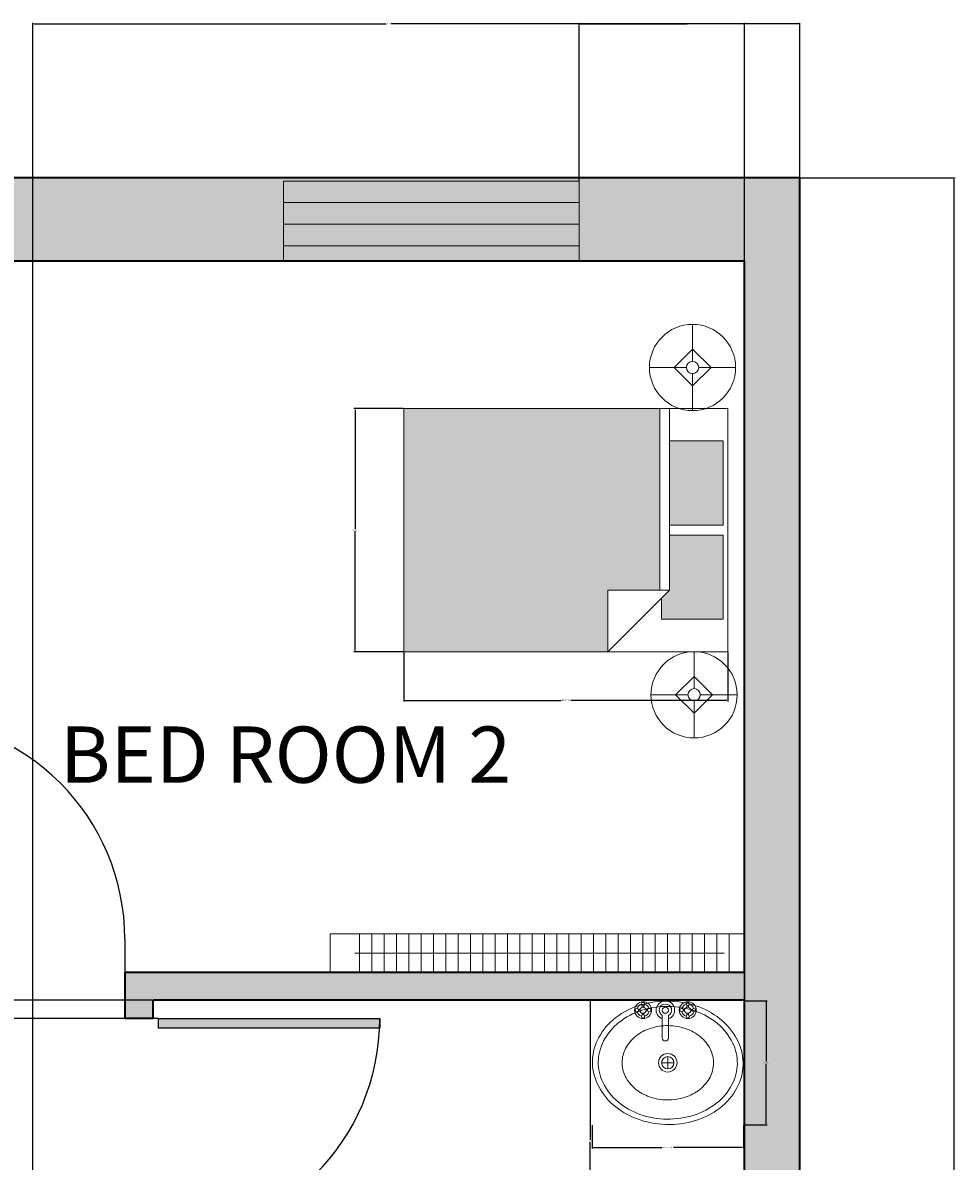
# Model space of a CAD drawing. Units: inches. Extents: x 1434 to 1845, y 1483 to 2014.
# Tile 11 of 11: x 1693 to 1845, y 1829 to 2014. Entities that reach past the tile are written whole.
import ezdxf

# ---------------------------------------------------------------- set-up
doc = ezdxf.new("R2010")
doc.units = ezdxf.units.IN
for name, color, linetype, lineweight in [('A-ANNO-DIMS', 2, 'Continuous', 18), ('A-AREA-IDEN', 7, 'Continuous', 25), ('A-DOOR', 3, 'Continuous', 25), ('A-FLOR-FIXT', 8, 'Continuous', 18), ('A-FLOR-FIXT-PATT', 8, 'Continuous', 13), ('A-FURN', 9, 'Continuous', 18), ('A-FURN-PATT', 9, 'Continuous', 13), ('A-GLAZ', 4, 'Continuous', 18), ('A-GLAZ-PATT', 9, 'Continuous', 13), ('A-WALL', 7, 'Continuous', 35), ('A-WALL-PATT', 8, 'Continuous', 13), ('E-LITE', 2, 'Continuous', 18)]:
    doc.layers.add(name, color=color, linetype=linetype, lineweight=lineweight)
doc.layers.add('A-DOOR-PATT', color=39, linetype='Continuous', lineweight=13, true_color=0x58382b)
doc.styles.get("Standard").update_dxf_attribs({"font": 'arial.ttf'})
doc.dimstyles.get("Standard").update_dxf_attribs({"dimtxt": 0.18, "dimasz": 0.18, "dimexe": 0.18, "dimexo": 0.0625, "dimgap": 0.09, "dimtad": 0, "dimtih": 1, "dimtoh": 1, "dimdec": 4, "dimzin": 0, "dimdsep": 46, "dimtxsty": 'Standard', "dimcen": 0.09, "dimadec": 0, "dimazin": 0, "dimtfac": 1, "dimtdec": 4, "dimtofl": 0, "dimtmove": 0, "dimatfit": 3, "dimfxl": 1, "dimtolj": 1, "dimtzin": 0, "dimarcsym": 0})

# ---------------------------------------------------------------- blocks, each defined once
blk = doc.blocks.new('*U3')
for p, q in [((0, 0), (0, -6)), ((40, 0), (40, -6))]:
    blk.add_line(p, q)
blk.add_lwpolyline([(0, 0), (0, 40), (1.75, 40), (1.75, 0)], close=True)
blk.add_arc((0, 0), 40, 0, 90)
blk = doc.blocks.new('Bed - Queen')
for p, q in [((0, -80.00003), (0, 0)), ((0, 0), (59.99999, 0)), ((59.99999, 0), (59.99999, -80.00003)), ((7.99999, -1.2), (28.79998, -1.2)), ((7.99999, -14.4), (7.99999, -1.2)), ((28.79998, -1.2), (28.79998, -14.4)), ((31.19999, -1.2), (51.99999, -1.2)), ((31.19999, -14.4), (31.19999, -1.2)), ((51.99999, -1.2), (51.99999, -16.4)), ((0, -14.4), (44.8, -14.4)), ((44.8, -16.8), (0, -16.8)), ((59.99999, -29.6), (44.8, -14.4)), ((44.8, -14.4), (44.8, -29.6)), ((51.99999, -16.4), (46.79936, -16.4)), ((44.8, -29.6), (59.99999, -29.6)), ((59.99999, -80.00003), (0, -80.00003))]:
    blk.add_line(p, q)
blk = doc.blocks.new('Lamp - Table')
for p, q in [((0, 7), (0, 1)), ((0, 3), (-3, 0)), ((3, 0), (0, 3)), ((-1, 0), (-7, 0)), ((-3, 0), (0, -3)), ((0, -3), (3, 0)), ((1, 0), (7, 0)), ((0, -1), (0, -7))]:
    blk.add_line(p, q)
for radius in [7, 1]:
    blk.add_circle((0, 0), radius)
blk = doc.blocks.new('Sink - Oval top')
for p, q in [((-1, 0), (1, 0)), ((0, 1), (0, -1))]:
    blk.add_line(p, q)
for points in [[(-12.23, 0.39, 0.117634), (-11.46, -3.36, 0.104469), (-8.88, -6.8, 0.090016), (-5.08, -9.07, 0.08192), (-0.32, -10.02, 0.08192), (4.49, -9.38, 0.090016), (8.42, -7.36, 0.104469), (11.22, -4.09, 0.117634), (12.23, -0.39, 0.117634), (11.46, 3.36, 0.104469), (8.88, 6.8, 0.090016), (5.08, 9.07, 0.08192), (0.32, 10.02, 0.08192), (-4.49, 9.38, 0.090016), (-8.42, 7.36, 0.104469), (-11.22, 4.09, 0.117634)], [(-11.29, 0.16, 0.118622), (-10.52, -3.25, 0.104678), (-8.07, -6.36, 0.089562), (-4.54, -8.37, 0.081185), (-0.13, -9.15, 0.081185), (4.3, -8.49, 0.089562), (7.89, -6.58, 0.104678), (10.42, -3.55, 0.118622), (11.29, -0.16, 0.118622), (10.52, 3.25, 0.104678), (8.07, 6.36, 0.089562), (4.54, 8.37, 0.081185), (0.13, 9.15, 0.081185), (-4.3, 8.49, 0.089562), (-7.89, 6.58, 0.104678), (-10.42, 3.55, 0.118622)], [(-7.42, 0.08, 0.118283), (-6.91, -2.17, 0.104607), (-5.29, -4.21, 0.089718), (-2.97, -5.53, 0.081436), (-0.07, -6.04, 0.081436), (2.84, -5.59, 0.089718), (5.2, -4.33, 0.104607), (6.86, -2.32, 0.118283), (7.42, -0.08, 0.118283), (6.91, 2.17, 0.104607), (5.29, 4.21, 0.089718), (2.97, 5.53, 0.081436), (0.07, 6.04, 0.081436), (-2.84, 5.59, 0.089718), (-5.2, 4.33, 0.104607), (-6.86, 2.32, 0.118283)]]:
    blk.add_lwpolyline(points, format="xyb", close=True)
for radius in [1.5, 1]:
    blk.add_circle((0, 0), radius)
blk = doc.blocks.new('Faucet - Bathroom top')
for p, q in [((-4.107, 0.125), (-4.375, 0.125)), ((-3.75, 0.4788), (-3.75, 0.75)), ((-3.5, 0.482), (-3.5, 0.75)), ((-3.1461, 0.125), (-2.875, 0.125)), ((3.143, 0.125), (2.875, 0.125)), ((3.5, 0.4788), (3.5, 0.75)), ((3.75, 0.482), (3.75, 0.75)), ((4.1039, 0.125), (4.375, 0.125)), ((-4.1039, -0.125), (-4.375, -0.125)), ((-3.75, -0.4821), (-3.75, -0.75)), ((-3.5, -0.4789), (-3.5, -0.75)), ((-3.143, -0.125), (-2.875, -0.125)), ((-0.5, -0.8639), (-0.5, -4.5)), ((0.5, -4.5), (0.5, -0.8631)), ((3.1461, -0.125), (2.875, -0.125)), ((3.5, -0.4821), (3.5, -0.75)), ((3.75, -0.4789), (3.75, -0.75)), ((4.107, -0.125), (4.375, -0.125))]:
    blk.add_line(p, q)
for centre, radius in [((-3.625, 0), 1.375), ((-4.625, 0), 0.2795), ((-3.625, 0), 0.5), ((-3.625, 1), 0.2795), ((-2.625, 0), 0.2795), ((0, 0), 0.5), ((3.625, 0), 1.375), ((2.625, 0), 0.2795), ((3.625, 0), 0.5), ((3.625, 1), 0.2795), ((4.625, 0), 0.2795), ((-3.625, -1), 0.2795), ((3.625, -1), 0.2795)]:
    blk.add_circle(centre, radius)
for centre, radius, start, end in [((-3.625, 0), 1, 105.2407, 164.2093), ((-3.625, 0), 1, 16.44125, 74.07887), ((0, 0), 1.5, 289.6514, 250.3603), ((0, 0), 1, 300.3431, 239.7554), ((3.625, 0), 1, 106.12, 164.0884), ((3.625, 0), 1, 16.23422, 73.90469), ((-3.625, 0), 1, 196.2342, 253.9047), ((-3.625, 0), 1, 286.12, 344.0884), ((3.625, 0), 1, 196.4413, 254.0789), ((3.625, 0), 1, 285.2407, 344.2093), ((0, -4.5), 0.5, 180, 0)]:
    blk.add_arc(centre, radius, start, end)
blk = doc.blocks.new('WIN-48IN-13IN')
for p, q in [((13, 48), (0, 48)), ((0, 48), (0, 12)), ((2.5, 48), (2.5, 0)), ((6, 48), (6, 0)), ((9.5, 48), (9.5, 0)), ((0, 12), (0, 0)), ((0, 0), (13, 0))]:
    blk.add_line(p, q)
blk.add_lwpolyline([(13, 48), (13, 0)], close=True)
blk = doc.blocks.new('*D22')
at = {"layer": 'A-ANNO-DIMS', "color": 0, "lineweight": -2, "transparency": 16777216}
for p, q in [((1755.17, 1911.37), (1755.17, 1903.35)), ((1807.81, 1911.37), (1807.81, 1903.35)), ((1755.35, 1903.53), (1780.67, 1903.53)), ((1807.63, 1903.53), (1782.31, 1903.53))]:
    blk.add_line(p, q, dxfattribs=at)
at = {"layer": 'A-ANNO-DIMS', "color": 0, "transparency": 16777216}
for points in [[(1755.35, 1903.56), (1755.35, 1903.5), (1755.17, 1903.53)], [(1807.63, 1903.56), (1807.63, 1903.5), (1807.81, 1903.53)]]:
    blk.add_solid(points, dxfattribs=at)
at = {"layer": 'Defpoints', "color": 0, "transparency": 16777216}
for p in [(1755.17, 1911.43), (1807.81, 1911.43), (1807.81, 1903.53)]:
    blk.add_point(p, dxfattribs=at)
at = {"layer": 'A-ANNO-DIMS', "color": 0, "transparency": 16777216, "insert": (1781.49, 1903.53), "char_height": 0.18, "attachment_point": 5}
blk.add_mtext('\\A1;BED 53 TYP.', dxfattribs=at)
blk = doc.blocks.new('*D23')
at = {"layer": 'A-ANNO-DIMS', "color": 0, "lineweight": -2, "transparency": 16777216}
for p, q in [((1755.1, 1950.91), (1747.09, 1950.91)), ((1747.27, 1950.73), (1747.27, 1931.35)), ((1747.27, 1911.61), (1747.27, 1930.99)), ((1755.1, 1911.43), (1747.09, 1911.43))]:
    blk.add_line(p, q, dxfattribs=at)
at = {"layer": 'A-ANNO-DIMS', "color": 0, "transparency": 16777216}
for points in [[(1747.24, 1950.73), (1747.3, 1950.73), (1747.27, 1950.91)], [(1747.24, 1911.61), (1747.3, 1911.61), (1747.27, 1911.43)]]:
    blk.add_solid(points, dxfattribs=at)
at = {"layer": 'Defpoints', "color": 0, "transparency": 16777216}
for p in [(1755.17, 1950.91), (1747.27, 1911.43), (1755.17, 1911.43)]:
    blk.add_point(p, dxfattribs=at)
at = {"layer": 'A-ANNO-DIMS', "color": 0, "transparency": 16777216, "insert": (1747.27, 1931.17), "char_height": 0.18, "attachment_point": 5}
blk.add_mtext('\\A1;39 TYP.', dxfattribs=at)
blk = doc.blocks.new('*D32')
at = {"layer": 'A-ANNO-DIMS', "color": 0, "lineweight": -2, "transparency": 16777216}
for p, q in [((1785.77, 1834.54), (1785.77, 1830.74)), ((1810.32, 1834.54), (1810.32, 1830.74)), ((1785.95, 1830.92), (1797.11, 1830.92)), ((1810.14, 1830.92), (1798.98, 1830.92))]:
    blk.add_line(p, q, dxfattribs=at)
at = {"layer": 'A-ANNO-DIMS', "color": 0, "transparency": 16777216}
for points in [[(1785.95, 1830.95), (1785.95, 1830.89), (1785.77, 1830.92)], [(1810.14, 1830.95), (1810.14, 1830.89), (1810.32, 1830.92)]]:
    blk.add_solid(points, dxfattribs=at)
at = {"layer": 'Defpoints', "color": 0, "transparency": 16777216}
for p in [(1785.77, 1834.61), (1810.32, 1834.61), (1810.32, 1830.92)]:
    blk.add_point(p, dxfattribs=at)
at = {"layer": 'A-ANNO-DIMS', "color": 0, "transparency": 16777216, "insert": (1798.04, 1830.92), "char_height": 0.18, "attachment_point": 5}
blk.add_mtext('\\A1;BASIN 25 TYP.', dxfattribs=at)
blk = doc.blocks.new('*D33')
at = {"layer": 'A-ANNO-DIMS', "color": 0, "lineweight": -2, "transparency": 16777216}
for p, q in [((1810.38, 1854.74), (1814.18, 1854.74)), ((1814, 1854.56), (1814, 1844.86)), ((1814, 1834.79), (1814, 1844.49)), ((1810.38, 1834.61), (1814.18, 1834.61))]:
    blk.add_line(p, q, dxfattribs=at)
at = {"layer": 'A-ANNO-DIMS', "color": 0, "transparency": 16777216}
for points in [[(1813.97, 1854.56), (1814.03, 1854.56), (1814, 1854.74)], [(1813.97, 1834.79), (1814.03, 1834.79), (1814, 1834.61)]]:
    blk.add_solid(points, dxfattribs=at)
at = {"layer": 'Defpoints', "color": 0, "transparency": 16777216}
for p in [(1810.32, 1854.74), (1814, 1854.74), (1810.32, 1834.61)]:
    blk.add_point(p, dxfattribs=at)
at = {"layer": 'A-ANNO-DIMS', "color": 0, "transparency": 16777216, "insert": (1814, 1844.68), "char_height": 0.18, "attachment_point": 5}
blk.add_mtext('\\A1;20 TYP.', dxfattribs=at)
blk = doc.blocks.new('*D55')
at = {"layer": 'A-ANNO-DIMS', "color": 0, "lineweight": -2, "transparency": 16777216}
for p, q in [((1819.54, 1988.36), (1844.68, 1988.36)), ((1844.5, 1988.18), (1844.5, 1748.54)), ((1844.5, 1508.54), (1844.5, 1748.17)), ((1819.54, 1508.36), (1844.68, 1508.36))]:
    blk.add_line(p, q, dxfattribs=at)
at = {"layer": 'A-ANNO-DIMS', "color": 0, "transparency": 16777216}
for points in [[(1844.47, 1988.18), (1844.53, 1988.18), (1844.5, 1988.36)], [(1844.47, 1508.54), (1844.53, 1508.54), (1844.5, 1508.36)]]:
    blk.add_solid(points, dxfattribs=at)
at = {"layer": 'Defpoints', "color": 0, "transparency": 16777216}
for p in [(1819.47, 1988.36), (1844.5, 1988.36), (1819.47, 1508.36)]:
    blk.add_point(p, dxfattribs=at)
at = {"layer": 'A-ANNO-DIMS', "color": 0, "transparency": 16777216, "insert": (1844.5, 1748.36), "char_height": 0.18, "attachment_point": 5}
blk.add_mtext('\\A1;480', dxfattribs=at)
blk = doc.blocks.new('*D58')
at = {"layer": 'A-ANNO-DIMS', "color": 0, "lineweight": -2, "transparency": 16777216}
for p, q in [((1670.97, 1974.79), (1670.97, 1483.15)), ((1810.47, 1974.79), (1810.47, 1483.15)), ((1671.15, 1483.33), (1740.34, 1483.33)), ((1810.29, 1483.33), (1741.11, 1483.33))]:
    blk.add_line(p, q, dxfattribs=at)
at = {"layer": 'A-ANNO-DIMS', "color": 0, "transparency": 16777216}
for points in [[(1671.15, 1483.36), (1671.15, 1483.3), (1670.97, 1483.33)], [(1810.29, 1483.36), (1810.29, 1483.3), (1810.47, 1483.33)]]:
    blk.add_solid(points, dxfattribs=at)
at = {"layer": 'Defpoints', "color": 0, "transparency": 16777216}
for p in [(1670.97, 1974.86), (1810.47, 1974.86), (1810.47, 1483.33)]:
    blk.add_point(p, dxfattribs=at)
at = {"layer": 'A-ANNO-DIMS', "color": 0, "transparency": 16777216, "insert": (1740.72, 1483.33), "char_height": 0.18, "attachment_point": 5}
blk.add_mtext('\\A1;139.5', dxfattribs=at)
blk = doc.blocks.new('*D67')
at = {"layer": 'A-ANNO-DIMS', "color": 0, "lineweight": -2, "transparency": 16777216}
for p, q in [((1694.97, 1517.42), (1694.97, 2013.56)), ((1695.15, 2013.38), (1752.34, 2013.38)), ((1810.29, 2013.38), (1753.11, 2013.38)), ((1810.47, 1517.42), (1810.47, 2013.56))]:
    blk.add_line(p, q, dxfattribs=at)
at = {"layer": 'A-ANNO-DIMS', "color": 0, "transparency": 16777216}
for points in [[(1695.15, 2013.41), (1695.15, 2013.35), (1694.97, 2013.38)], [(1810.29, 2013.41), (1810.29, 2013.35), (1810.47, 2013.38)]]:
    blk.add_solid(points, dxfattribs=at)
at = {"layer": 'Defpoints', "color": 0, "transparency": 16777216}
for p in [(1810.47, 2013.38), (1694.97, 1517.36), (1810.47, 1517.36)]:
    blk.add_point(p, dxfattribs=at)
at = {"layer": 'A-ANNO-DIMS', "color": 0, "transparency": 16777216, "insert": (1752.72, 2013.38), "char_height": 0.18, "attachment_point": 5}
blk.add_mtext('\\A1;115.5', dxfattribs=at)
blk = doc.blocks.new('*D75')
at = {"layer": 'A-ANNO-DIMS', "color": 0, "lineweight": -2, "transparency": 16777216}
for p, q in [((1783.65, 1987.92), (1783.65, 2013.56)), ((1783.83, 2013.38), (1801.17, 2013.38)), ((1819.29, 2013.38), (1801.96, 2013.38)), ((1819.47, 1988.42), (1819.47, 2013.56))]:
    blk.add_line(p, q, dxfattribs=at)
at = {"layer": 'A-ANNO-DIMS', "color": 0, "transparency": 16777216}
for points in [[(1783.83, 2013.41), (1783.83, 2013.35), (1783.65, 2013.38)], [(1819.29, 2013.41), (1819.29, 2013.35), (1819.47, 2013.38)]]:
    blk.add_solid(points, dxfattribs=at)
at = {"layer": 'Defpoints', "color": 0, "transparency": 16777216}
for p in [(1819.47, 2013.38), (1783.65, 1987.86), (1819.47, 1988.36)]:
    blk.add_point(p, dxfattribs=at)
at = {"layer": 'A-ANNO-DIMS', "color": 0, "transparency": 16777216, "insert": (1801.56, 2013.38), "char_height": 0.18, "attachment_point": 5}
blk.add_mtext('\\A1;35.82', dxfattribs=at)
blk = doc.blocks.new('*D79')
at = {"layer": 'A-ANNO-DIMS', "color": 0, "lineweight": -2, "transparency": 16777216}
for p, q in [((1810.41, 1854.86), (1785.27, 1854.86)), ((1785.45, 1854.68), (1785.45, 1832.19)), ((1785.45, 1809.35), (1785.45, 1831.83)), ((1810.41, 1809.17), (1785.27, 1809.17))]:
    blk.add_line(p, q, dxfattribs=at)
at = {"layer": 'A-ANNO-DIMS', "color": 0, "transparency": 16777216}
for points in [[(1785.42, 1854.68), (1785.48, 1854.68), (1785.45, 1854.86)], [(1785.42, 1809.35), (1785.48, 1809.35), (1785.45, 1809.17)]]:
    blk.add_solid(points, dxfattribs=at)
at = {"layer": 'Defpoints', "color": 0, "transparency": 16777216}
for p in [(1785.45, 1854.86), (1810.47, 1854.86), (1810.47, 1809.17)]:
    blk.add_point(p, dxfattribs=at)
at = {"layer": 'A-ANNO-DIMS', "color": 0, "transparency": 16777216, "insert": (1785.45, 1832.01), "char_height": 0.18, "attachment_point": 5}
blk.add_mtext('\\A1;45.69', dxfattribs=at)
blk = doc.blocks.new('*D90')
at = {"layer": 'A-ANNO-DIMS', "color": 0, "lineweight": -2, "transparency": 16777216}
for p, q in [((1714.41, 1854.86), (1689.27, 1854.86)), ((1689.45, 1854.68), (1689.45, 1853.54)), ((1689.45, 1852.04), (1689.45, 1853.17)), ((1714.41, 1851.86), (1689.27, 1851.86))]:
    blk.add_line(p, q, dxfattribs=at)
at = {"layer": 'A-ANNO-DIMS', "color": 0, "transparency": 16777216}
for points in [[(1689.42, 1854.68), (1689.48, 1854.68), (1689.45, 1854.86)], [(1689.42, 1852.04), (1689.48, 1852.04), (1689.45, 1851.86)]]:
    blk.add_solid(points, dxfattribs=at)
at = {"layer": 'Defpoints', "color": 0, "transparency": 16777216}
for p in [(1689.45, 1854.86), (1714.47, 1854.86), (1714.47, 1851.86)]:
    blk.add_point(p, dxfattribs=at)
at = {"layer": 'A-ANNO-DIMS', "color": 0, "transparency": 16777216, "insert": (1689.45, 1853.36), "char_height": 0.18, "attachment_point": 5}
blk.add_mtext('\\A1;3', dxfattribs=at)

msp = doc.modelspace()

# ---------------------------------------------------------------- hatches: boundary and pattern name
at = {"layer": 'A-DOOR-PATT'}
h = msp.add_hatch(color=256, dxfattribs=at)
h.dxf.hatch_style = 1
h.paths.add_polyline_path([(1611.5864, 1583.2737), (1575.6681, 1583.2737, 0.01094143), (1575.7025, 1581.7022), (1611.5864, 1581.7022)])
h.paths.add_polyline_path([(1621.4742, 1547.3553), (1616.9742, 1547.3553), (1616.9742, 1544.3553), (1621.4742, 1544.3553)])
h.paths.add_polyline_path([(1635.0456, 1558.627, 0.01094143), (1633.4742, 1558.6614), (1633.4742, 1522.7431), (1635.0456, 1522.7431)])
h.paths.add_polyline_path([(1633.4742, 1517.3553), (1630.4742, 1517.3553), (1630.4742, 1508.3553), (1633.4742, 1508.3553)])
h.paths.add_polyline_path([(1672.8212, 1517.3553), (1669.8212, 1517.3553), (1669.8212, 1508.3553), (1672.8212, 1508.3553)])
h.paths.add_polyline_path([(1613.8925, 1724.9676), (1612.3211, 1724.9676), (1612.3211, 1689.0836, 0.01094143), (1613.8925, 1689.0492)])
h.paths.add_polyline_path([(1789.3925, 1684.9726), (1753.4742, 1684.9726), (1753.4742, 1683.4011), (1789.3925, 1683.4011)])
h.paths.add_polyline_path([(1792.4742, 1679.5848), (1789.4742, 1679.5848), (1789.4742, 1675.0848), (1792.4742, 1675.0848)])
h.paths.add_polyline_path([(1563.5864, 1851.7737), (1527.6681, 1851.7737, 0.01094143), (1527.7025, 1850.2022), (1563.5864, 1850.2022)])
h.paths.add_polyline_path([(1609.3925, 1900.6614, 0.01094143), (1607.8211, 1900.627), (1607.8211, 1864.7431), (1609.3925, 1864.7431)])
h.paths.add_polyline_path([(1675.5456, 1900.627, 0.01094143), (1673.9742, 1900.6614), (1673.9742, 1864.7431), (1675.5456, 1864.7431)])
h.paths.add_polyline_path([(1751.2803, 1851.8553), (1715.3619, 1851.8553), (1715.3619, 1850.2839), (1751.2459, 1850.2839, 0.01094143)])
at = {"layer": 'A-FLOR-FIXT-PATT'}
h = msp.add_hatch(dxfattribs=at)
h.set_pattern_fill('ANSI31', color=256, scale=0.629921, angle=45, style=0)
h.paths.add_polyline_path([(1746.2071, 1859.3553), (1808.2071, 1859.3553), (1808.2071, 1865.5944), (1746.2071, 1865.5944)])
at = {"layer": 'A-FURN-PATT'}
h = msp.add_hatch(color=256, dxfattribs=at)
h.dxf.hatch_style = 1
h.paths.add_polyline_path([(1528.2614, 1944.8381), (1495.0961, 1944.8381), (1495.0961, 1934.8359), (1486.6731, 1934.8359), (1486.6731, 1905.3556), (1528.2614, 1905.3556)])
h.paths.add_polyline_path([(1796.7541, 1950.9116), (1755.1658, 1950.9116), (1755.1658, 1911.4291), (1788.3311, 1911.4291), (1788.3311, 1921.4313), (1796.7541, 1921.4313)])
h.paths.add_polyline_path([(1529.423, 1679.282), (1496.2577, 1679.282), (1496.2577, 1669.2798), (1487.8347, 1669.2798), (1487.8347, 1639.7996), (1529.423, 1639.7996)])
h.paths.add_polyline_path([(1486.2554, 1669.2798), (1487.5715, 1670.5959), (1487.5715, 1674.0177), (1477.5693, 1674.0177), (1477.5693, 1660.3304), (1486.2554, 1660.3304)])
h.paths.add_polyline_path([(1486.2554, 1658.7511), (1477.5693, 1658.7511), (1477.5693, 1645.0639), (1486.2554, 1645.0639)])
h.paths.add_polyline_path([(1807.0195, 1930.3807), (1798.3334, 1930.3807), (1798.3334, 1921.4313), (1797.0173, 1920.1152), (1797.0173, 1916.6934), (1807.0195, 1916.6934)])
h.paths.add_polyline_path([(1807.0195, 1945.6472), (1798.3334, 1945.6472), (1798.3334, 1931.96), (1807.0195, 1931.96)])
h.paths.add_polyline_path([(1485.0938, 1934.8359), (1486.4099, 1936.152), (1486.4099, 1939.5738), (1476.4077, 1939.5738), (1476.4077, 1925.8865), (1485.0938, 1925.8865)])
h.paths.add_polyline_path([(1485.0938, 1924.3072), (1476.4077, 1924.3072), (1476.4077, 1910.62), (1485.0938, 1910.62)])
at = {"layer": 'A-GLAZ-PATT'}
h = msp.add_hatch(color=256, dxfattribs=at)
h.dxf.hatch_style = 1
h.set_gradient(color1=(0, 0, 255), color2=(255, 255, 0), name='INVCURVED')
h.paths.add_polyline_path([(1783.6549, 1987.8553), (1735.6549, 1987.8553), (1735.6549, 1984.3553), (1783.6549, 1984.3553)])
h.paths.add_polyline_path([(1783.6549, 1984.3553), (1735.6549, 1984.3553), (1735.6549, 1980.8553), (1783.6549, 1980.8553)])
h.paths.add_polyline_path([(1783.6549, 1980.8553), (1735.6549, 1980.8553), (1735.6549, 1977.3553), (1783.6549, 1977.3553)])
h.paths.add_polyline_path([(1783.6549, 1977.3553), (1735.6549, 1977.3553), (1735.6549, 1974.8553), (1771.6549, 1974.8553), (1783.6549, 1974.8553)])
at = {"layer": 'A-WALL-PATT'}
h = msp.add_hatch(color=256, dxfattribs=at)
h.dxf.hatch_style = 1
h.paths.add_polyline_path([(1472.9742, 1730.3553), (1577.9742, 1730.3553), (1577.9742, 1734.8553), (1573.4742, 1734.8553), (1573.4742, 1815.8553), (1568.9742, 1815.8553), (1568.9742, 1734.8553), (1472.9742, 1734.8553), (1472.9742, 1770.1951), (1459.9742, 1770.1951), (1459.9742, 1782.1951), (1459.9742, 1818.1951), (1472.9742, 1818.1951), (1472.9742, 1854.8553), (1568.9742, 1854.8553), (1568.9742, 1851.8553), (1573.4742, 1851.8553), (1573.4742, 1854.8553), (1573.4742, 1859.3553), (1472.9742, 1859.3553), (1472.9742, 1899.9369), (1459.9742, 1899.9369), (1459.9742, 1911.9369), (1459.9742, 1947.9369), (1472.9742, 1947.9369), (1472.9742, 1974.8553), (1513.9785, 1974.8553), (1513.9785, 1987.8553), (1561.9785, 1987.8553), (1561.9785, 1974.8553), (1612.4742, 1974.8553), (1612.4742, 1859.3553), (1609.4742, 1859.3553), (1609.4742, 1854.8553), (1616.9742, 1854.8553), (1616.9742, 1910.3553), (1625.153, 1910.3553), (1625.153, 1914.8553), (1616.9742, 1914.8553), (1616.9742, 1988.3553), (1459.4742, 1988.3553), (1459.4742, 1508.3553), (1630.4742, 1508.3553), (1630.4742, 1517.3553), (1472.9742, 1517.3553), (1472.9742, 1586.3553), (1616.9742, 1586.3553), (1616.9742, 1583.3553), (1621.4742, 1583.3553), (1621.4742, 1586.3553), (1621.4742, 1734.8553), (1616.9742, 1734.8553), (1613.9742, 1734.8553), (1613.9742, 1730.3553), (1616.9742, 1730.3553), (1616.9742, 1590.8553), (1472.9742, 1590.8553), (1472.9742, 1635.7299), (1459.9742, 1635.7299), (1459.9742, 1647.7299), (1459.9742, 1683.7299), (1472.9742, 1683.7299)])
h.paths.add_polyline_path([(1819.4742, 1773.1667), (1810.4742, 1773.1667), (1810.4742, 1734.8553), (1714.4742, 1734.8553), (1714.4742, 1815.8553), (1709.9742, 1815.8553), (1709.9742, 1730.3553), (1745.9742, 1730.3553), (1745.9742, 1675.0848), (1753.4742, 1675.0848), (1753.4742, 1679.5848), (1750.4742, 1679.5848), (1750.4742, 1730.3553), (1810.4742, 1730.3553), (1810.4742, 1679.5848), (1792.4742, 1679.5848), (1792.4742, 1675.0848), (1810.4742, 1675.0848), (1810.4742, 1517.3553), (1775.1129, 1517.3553), (1775.1129, 1508.3553), (1819.4742, 1508.3553)])
h.paths.add_polyline_path([(1739.1129, 1517.3553), (1694.9742, 1517.3553), (1694.9742, 1730.3553), (1690.4742, 1730.3553), (1690.4742, 1517.3553), (1678.4742, 1517.3553), (1675.4742, 1517.3553), (1672.8212, 1517.3553), (1672.8212, 1508.3553), (1678.4742, 1508.3553), (1739.1129, 1508.3553)])
h.paths.add_polyline_path([(1735.6549, 1987.8553), (1783.6549, 1987.8553), (1783.6549, 1974.8553), (1810.4742, 1974.8553), (1810.4742, 1859.3553), (1709.9742, 1859.3553), (1709.9742, 1854.8553), (1709.9742, 1851.8553), (1714.4742, 1851.8553), (1714.4742, 1854.8553), (1810.4742, 1854.8553), (1810.4742, 1809.1667), (1819.4742, 1809.1667), (1819.4742, 1988.3553), (1666.4742, 1988.3553), (1666.4742, 1914.8553), (1661.1087, 1914.8553), (1661.1087, 1910.3553), (1666.4742, 1910.3553), (1666.4742, 1854.8553), (1673.9742, 1854.8553), (1673.9742, 1859.3553), (1670.9742, 1859.3553), (1670.9742, 1974.8553), (1735.6549, 1974.8553)])

# ---------------------------------------------------------------- linework, layer by layer
at = {"layer": 'A-FLOR-FIXT'}
for p, q in [((1810.4742, 1865.5944), (1743.2071, 1865.5944)), ((1743.2071, 1865.5944), (1743.2071, 1859.3553)), ((1743.2071, 1865.5944), (1743.2071, 1859.3553)), ((1743.2071, 1865.5944), (1743.2071, 1859.3553)), ((1810.4742, 1859.3553), (1810.4742, 1865.5944)), ((1747.2071, 1862.4748), (1807.2071, 1862.4748)), ((1743.2071, 1859.3553), (1810.4742, 1859.3553))]:
    msp.add_line(p, q, dxfattribs=at)
at = {"layer": 'A-WALL'}
for p, q in [((1810.4742, 1974.8553), (1670.9742, 1974.8553)), ((1810.4742, 1859.3553), (1810.4742, 1974.8553)), ((1810.4742, 1859.3553), (1709.9742, 1859.3553)), ((1709.9742, 1854.8553), (1709.9742, 1859.3553)), ((1709.9742, 1851.8553), (1709.9742, 1859.3553)), ((1810.4742, 1854.8553), (1714.4742, 1854.8553)), ((1714.4742, 1851.8553), (1714.4742, 1854.8553)), ((1810.4742, 1734.8553), (1810.4742, 1854.8553)), ((1714.4742, 1851.8553), (1709.9742, 1851.8553))]:
    msp.add_line(p, q, dxfattribs=at)
msp.add_lwpolyline([(1678.4742, 1508.3553), (1819.4742, 1508.3553), (1819.4742, 1988.3553), (1459.4742, 1988.3553), (1459.4742, 1508.3553), (1630.4742, 1508.3553)], dxfattribs=at)

# ---------------------------------------------------------------- block references
at = {"layer": 'A-DOOR', "xscale": 0.8979587755198419, "yscale": 0.8979587755198419, "zscale": 0.8979587755198419}
msp.add_blockref('*U3', (1673.9742, 1864.7431), dxfattribs=at)
at = {"layer": 'A-DOOR', "xscale": 0.8979587755198419, "yscale": 0.8979587755198419, "zscale": 0.8979587755198419, "rotation": 270}
msp.add_blockref('*U3', (1715.3619, 1851.8553), dxfattribs=at)
at = {"layer": 'A-FLOR-FIXT'}
for name, p in [('Sink - Oval top', (1798.0428, 1844.6752)), ('Faucet - Bathroom top', (1797.6544, 1853.2166))]:
    msp.add_blockref(name, p, dxfattribs=at)
at = {"layer": 'A-FURN', "xscale": 0.6580416786709006, "yscale": 0.6580416786709006, "zscale": 0.6580416786709006, "rotation": 270}
msp.add_blockref('Bed - Queen', (1807.8092, 1950.9116), dxfattribs=at)
at = {"layer": 'A-GLAZ', "rotation": 90.00000000000058}
msp.add_blockref('WIN-48IN-13IN', (1783.6549, 1974.8553), dxfattribs=at)
at = {"layer": 'E-LITE'}
for p in [(1802.0562, 1957.5806), (1802.3099, 1904.4291)]:
    msp.add_blockref('Lamp - Table', p, dxfattribs=at)

# ---------------------------------------------------------------- texts
at = {"layer": 'A-AREA-IDEN'}
msp.add_text('BED ROOM 2', height=9.14668, dxfattribs=at).set_placement((1699.3723, 1890.1412))

# ---------------------------------------------------------------- dimensions: what is measured, and where the dimension line sits
at = {"layer": 'A-ANNO-DIMS'}
for base, p1, p2, override, picture, middle in [((1810.4742, 2013.3803), (1694.9742, 1517.3553), (1810.4742, 1517.3553), {"dimdec": 1, "dimlfac": 1, "dimrnd": 0, "dimzin": 0, "dimdsep": 46, "dimlunit": 2}, '*D67', (1752.7242, 2013.3803)), ((1819.4742, 2013.3803), (1783.6549, 1987.8553), (1819.4742, 1988.3553), {"dimdec": 2, "dimlfac": 1, "dimrnd": 0, "dimzin": 0, "dimdsep": 46, "dimlunit": 2}, '*D75', (1801.5646, 2013.3803)), ((1810.4742, 1483.3303), (1670.9742, 1974.8553), (1810.4742, 1974.8553), {"dimdec": 1, "dimlfac": 1, "dimrnd": 0, "dimzin": 0, "dimdsep": 46, "dimlunit": 2}, '*D58', (1740.7242, 1483.3303))]:
    dim = msp.add_linear_dim(base=base, p1=p1, p2=p2, dimstyle='Standard', override=override, dxfattribs=at)
    dim.commit()
    dim.dimension.update_dxf_attribs({"geometry": picture, "text_midpoint": middle})
for base, p1, p2, override, picture, middle in [((1844.4992, 1988.3553), (1819.4742, 1508.3553), (1819.4742, 1988.3553), {"dimdec": 0, "dimlfac": 1, "dimrnd": 0, "dimzin": 0, "dimdsep": 46, "dimlunit": 2}, '*D55', (1844.4992, 1748.3553)), ((1689.4492, 1854.8553), (1714.4742, 1851.8553), (1714.4742, 1854.8553), {"dimdec": 0, "dimlfac": 1, "dimrnd": 0, "dimzin": 0, "dimdsep": 46, "dimlunit": 2}, '*D90', (1689.4492, 1853.3553)), ((1785.4492, 1854.8553), (1810.4742, 1809.1667), (1810.4742, 1854.8553), {"dimdec": 2, "dimlfac": 1, "dimrnd": 0, "dimzin": 0, "dimdsep": 46, "dimlunit": 2}, '*D79', (1785.4492, 1832.011))]:
    dim = msp.add_linear_dim(base=base, p1=p1, p2=p2, angle=90, dimstyle='Standard', override=override, dxfattribs=at)
    dim.commit()
    dim.dimension.update_dxf_attribs({"geometry": picture, "text_midpoint": middle})
for base, p1, p2, angle, picture, middle in [((1747.2693, 1911.4291), (1755.1658, 1950.9116), (1755.1658, 1911.4291), 270, '*D23', (1747.2693, 1931.1703)), ((1814.0009, 1854.7435), (1810.3182, 1834.6069), (1810.3182, 1854.7435), 90, '*D33', (1814.0009, 1844.6752))]:
    dim = msp.add_linear_dim(base=base, p1=p1, p2=p2, angle=angle, text='<> TYP.', dimstyle='Standard', override={"dimdec": 0, "dimlfac": 1, "dimrnd": 0, "dimzin": 0, "dimdsep": 46, "dimlunit": 2}, dxfattribs=at)
    dim.commit()
    dim.dimension.update_dxf_attribs({"geometry": picture, "text_midpoint": middle})
for base, p1, p2, text, picture, middle in [((1807.8092, 1903.5326), (1755.1658, 1911.4291), (1807.8092, 1911.4291), 'BED <> TYP.', '*D22', (1781.4875, 1903.5326)), ((1810.3182, 1830.9242), (1785.7673, 1834.6069), (1810.3182, 1834.6069), 'BASIN <> TYP.', '*D32', (1798.0428, 1830.9242))]:
    dim = msp.add_linear_dim(base=base, p1=p1, p2=p2, text=text, dimstyle='Standard', override={"dimdec": 0, "dimlfac": 1, "dimrnd": 0, "dimzin": 0, "dimdsep": 46, "dimlunit": 2}, dxfattribs=at)
    dim.commit()
    dim.dimension.update_dxf_attribs({"geometry": picture, "text_midpoint": middle})

doc.saveas('drawing.dxf')
